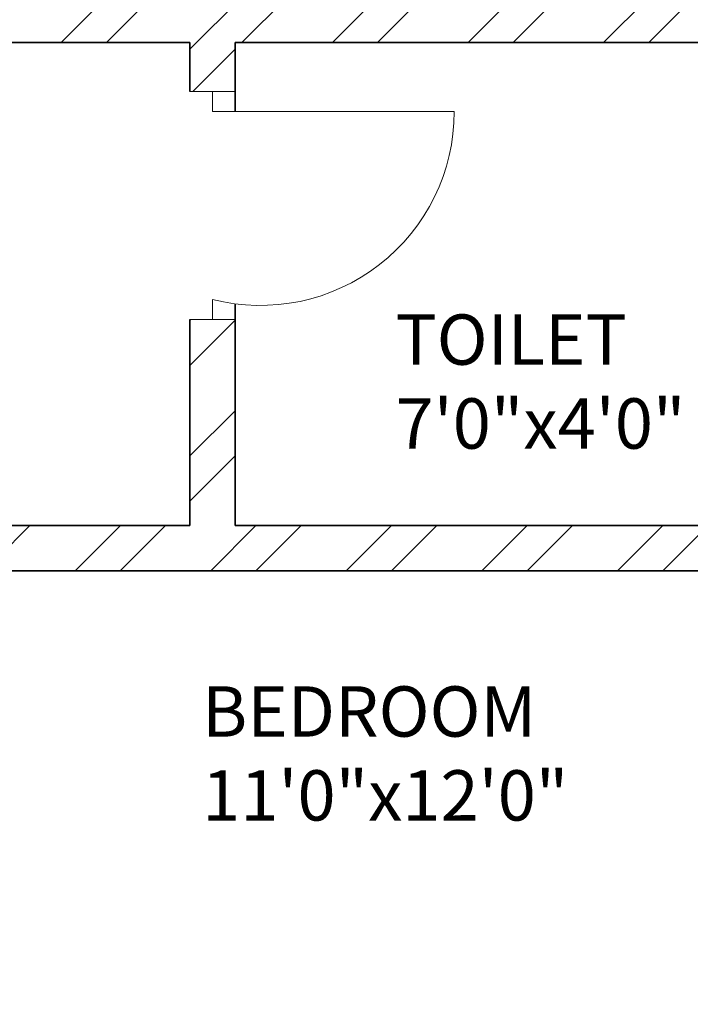
# Model space of a CAD drawing. Units: inches. Extents: x 1962 to 2771, y 1245 to 2660.
# Tile 78 of 114: x 2551 to 2618, y 2082 to 2180. Entities that reach past the tile are written whole.
import ezdxf

# ---------------------------------------------------------------- set-up
doc = ezdxf.new("R2010")
doc.units = ezdxf.units.IN
for name, color, linetype, lineweight in [('A-ANNO-DIMS', 2, 'Continuous', 18), ('A-AREA-IDEN', 7, 'Continuous', 18), ('A-DOOR', 3, 'Continuous', 18), ('A-WALL', 7, 'Continuous', 35), ('A-WALL-PATT', 252, 'Continuous', 13)]:
    doc.layers.add(name, color=color, linetype=linetype, lineweight=lineweight)
doc.styles.get("Standard").update_dxf_attribs({"font": 'arial.ttf'})
doc.dimstyles.get("Standard").update_dxf_attribs({"dimtxt": 0.18, "dimasz": 0.18, "dimexe": 0.18, "dimexo": 0.0625, "dimgap": 0.09, "dimtad": 0, "dimtih": 1, "dimtoh": 1, "dimdec": 4, "dimzin": 0, "dimdsep": 46, "dimtxsty": 'Standard', "dimcen": 0.09, "dimadec": 0, "dimazin": 0, "dimtfac": 1, "dimtdec": 4, "dimtofl": 0, "dimtmove": 0, "dimatfit": 3, "dimfxl": 1, "dimtolj": 1, "dimtzin": 0, "dimarcsym": 0})

# ---------------------------------------------------------------- blocks, each defined once
blk = doc.blocks.new('*D40')
at = {"layer": 'A-ANNO-DIMS', "color": 0, "lineweight": -2, "transparency": 16777216}
for p, q in [((2072.02, 2033.906), (2072.02, 2583.474)), ((2072.2, 2583.294), (2366.02, 2583.294)), ((2660.627, 2583.294), (2366.808, 2583.294)), ((2660.807, 2524.406), (2660.807, 2583.474))]:
    blk.add_line(p, q, dxfattribs=at)
at = {"layer": 'A-ANNO-DIMS', "color": 0, "transparency": 16777216}
for points in [[(2072.2, 2583.324), (2072.2, 2583.264), (2072.02, 2583.294)], [(2660.627, 2583.324), (2660.627, 2583.264), (2660.807, 2583.294)]]:
    blk.add_solid(points, dxfattribs=at)
at = {"layer": 'Defpoints', "color": 0, "transparency": 16777216}
for p in [(2660.807, 2583.294), (2660.807, 2524.344), (2072.02, 2033.844)]:
    blk.add_point(p, dxfattribs=at)
at = {"layer": 'A-ANNO-DIMS', "color": 0, "transparency": 16777216, "insert": (2366.414, 2583.294), "char_height": 0.18, "attachment_point": 5}
blk.add_mtext('\\A1;588.8', dxfattribs=at)

msp = doc.modelspace()

# ---------------------------------------------------------------- hatches: boundary and pattern name
at = {"layer": 'A-WALL-PATT'}
h = msp.add_hatch(dxfattribs=at)
h.set_pattern_fill('ANSI32', color=256)
h.paths.add_polyline_path([(2090.8074, 2467.3437), (2141.6481, 2467.3437), (2141.6481, 2469.5937), (2141.6481, 2471.8437), (2086.3074, 2471.8437), (2086.3074, 2422.5333), (2090.8074, 2422.5333)])
h.paths.add_polyline_path([(2282.7664, 2471.8437), (2204.8982, 2471.8437), (2204.8982, 2467.3437), (2234.8074, 2467.3437), (2234.8074, 2311.3437), (2228.7492, 2311.3437), (2228.7492, 2306.8437), (2234.8074, 2306.8437), (2331.9227, 2306.8437), (2331.9227, 2309.0937), (2331.9227, 2311.3437), (2239.3074, 2311.3437), (2239.3074, 2467.3437), (2282.7664, 2467.3437), (2282.7664, 2469.5937)])
h.paths.add_polyline_path([(2471.4531, 2519.8437), (2552.011, 2519.8437), (2564.3996, 2519.8437), (2564.3996, 2511.1389), (2568.8996, 2511.1389), (2568.8996, 2524.3437), (2466.9531, 2524.3437), (2466.9531, 2471.8437), (2450.0749, 2471.8437), (2446.4672, 2471.8437), (2446.4672, 2467.3437), (2450.0749, 2467.3437), (2475.9988, 2467.3437), (2475.9988, 2469.5937), (2475.9988, 2471.8437), (2471.4531, 2471.8437)])
h.paths.add_polyline_path([(2575.2231, 2469.5937), (2575.2231, 2471.8437), (2568.8996, 2471.8437), (2568.8996, 2487.1389), (2564.3996, 2487.1389), (2564.3996, 2471.8437), (2556.511, 2471.8437), (2499.2904, 2471.8437), (2499.2904, 2467.3437), (2507.8074, 2467.3437), (2507.8074, 2311.3437), (2414.863, 2311.3437), (2414.863, 2306.8437), (2512.3074, 2306.8437), (2517.0114, 2306.8437), (2517.0114, 2309.0937), (2517.0114, 2311.3437), (2512.3074, 2311.3437), (2512.3074, 2467.3437), (2575.2231, 2467.3437)])
h.paths.add_polyline_path([(2660.8074, 2471.8437), (2600.9602, 2471.8437), (2600.9602, 2467.3437), (2656.3074, 2467.3437), (2656.3074, 2432.5704), (2660.8074, 2432.5704)])
h.paths.add_polyline_path([(2660.8074, 2372.5704), (2656.3074, 2372.5704), (2656.3074, 2311.3437), (2600.276, 2311.3437), (2600.276, 2309.0937), (2600.276, 2306.8437), (2656.3074, 2306.8437), (2656.3074, 2296.2593), (2660.8074, 2296.2593)])
h.paths.add_polyline_path([(2572.3074, 2306.8437), (2577.1385, 2306.8437), (2577.1385, 2311.3437), (2551.082, 2311.3437), (2551.082, 2306.8437), (2567.8074, 2306.8437), (2567.8074, 2258.8437), (2540.0574, 2258.8437), (2540.0574, 2256.5937), (2540.0574, 2254.3437), (2567.8074, 2254.3437), (2656.3074, 2254.3437), (2656.3074, 2236.9085), (2660.8074, 2236.9085), (2660.8074, 2272.2593), (2656.3074, 2272.2593), (2656.3074, 2258.8437), (2572.3074, 2258.8437)])
h.paths.add_polyline_path([(2512.3074, 2254.3437), (2518.8716, 2254.3437), (2518.8716, 2256.5937), (2518.8716, 2258.8437), (2507.8074, 2258.8437), (2507.8074, 2177.8437), (2567.8074, 2177.8437), (2567.8074, 2172.9628), (2572.3074, 2172.9628), (2572.3074, 2177.8437), (2656.3074, 2177.8437), (2656.3074, 2166.4846), (2660.8074, 2166.4846), (2660.8074, 2200.9085), (2656.3074, 2200.9085), (2656.3074, 2182.3437), (2512.3074, 2182.3437)])
h.paths.add_polyline_path([(2656.3074, 2129.8437), (2572.3074, 2129.8437), (2572.3074, 2150.3044), (2570.0574, 2150.3044), (2567.8074, 2150.3044), (2567.8074, 2129.8437), (2507.8074, 2129.8437), (2507.8074, 2116.3027), (2510.0574, 2116.3027), (2512.3074, 2116.3027), (2512.3074, 2125.3437), (2567.8074, 2125.3437), (2572.3074, 2125.3437), (2656.3074, 2125.3437)])
h.paths.add_polyline_path([(2090.8074, 2362.5333), (2086.3074, 2362.5333), (2086.3074, 2298.6242), (2090.8074, 2298.6242), (2090.8074, 2306.8437), (2174.8074, 2306.8437), (2174.8074, 2286.4178), (2179.3074, 2286.4178), (2179.3074, 2306.8437), (2192.8641, 2306.8437), (2192.8641, 2309.0937), (2192.8641, 2311.3437), (2090.8074, 2311.3437)])
h.paths.add_polyline_path([(2209.156, 2258.8437), (2179.3074, 2258.8437), (2179.3074, 2263.2236), (2177.0574, 2263.2236), (2174.8074, 2263.2236), (2174.8074, 2258.8437), (2090.8074, 2258.8437), (2090.8074, 2274.6242), (2086.3074, 2274.6242), (2086.3074, 2238.2967), (2088.5574, 2238.2967), (2090.8074, 2238.2967), (2090.8074, 2254.3437), (2209.156, 2254.3437)])
h.paths.add_polyline_path([(2090.8074, 2177.8437), (2234.8074, 2177.8437), (2234.8074, 2173.1428), (2239.3074, 2173.1428), (2239.3074, 2258.8437), (2230.8442, 2258.8437), (2230.8442, 2256.5937), (2230.8442, 2254.3437), (2234.8074, 2254.3437), (2234.8074, 2182.3437), (2090.8074, 2182.3437), (2090.8074, 2202.2967), (2086.3074, 2202.2967), (2086.3074, 2140.0389), (2090.8074, 2140.0389)])
h.paths.add_polyline_path([(2090.8074, 2080.0389), (2086.3074, 2080.0389), (2086.3074, 2033.8437), (2090.8074, 2033.8437)], flags=17)
h.paths.add_polyline_path([(2244.9405, 2033.8437), (2239.3074, 2033.8437), (2239.3074, 2142.0665), (2237.2592, 2142.0665), (2234.8074, 2142.0665), (2234.8074, 2033.8437), (2090.8074, 2033.8437), (2076.5204, 2033.8437), (2072.0204, 2033.8437), (2072.0204, 2000.4493), (2076.5204, 2000.4493), (2076.5204, 2029.3437), (2090.8074, 2029.3437), (2244.9405, 2029.3437), (2244.9405, 2031.5937)])
h.paths.add_polyline_path([(2234.8074, 1933.3437), (2076.5204, 1933.3437), (2076.5204, 1952.4493), (2074.2704, 1952.4493), (2072.0204, 1952.4493), (2072.0204, 1933.3437), (2072.0204, 1928.8437), (2234.8074, 1928.8437)])
h.paths.add_polyline_path([(2090.8074, 1928.8437), (2086.3074, 1928.8437), (2086.3074, 1906.5013), (2090.8074, 1906.5013)])
h.paths.add_polyline_path([(2090.8074, 1846.5013), (2086.3074, 1846.5013), (2086.3074, 1769.9917), (2088.5574, 1769.9917), (2090.8074, 1769.9917), (2090.8074, 1780.3437), (2234.8074, 1780.3437), (2234.8074, 1708.3437), (2230.3764, 1708.3437), (2230.3764, 1703.8437), (2239.3074, 1703.8437), (2239.3074, 1792.6669), (2237.0574, 1792.6669), (2234.8074, 1792.6669), (2234.8074, 1784.8437), (2090.8074, 1784.8437)])
h.paths.add_polyline_path([(2239.3074, 1928.8437), (2244.9405, 1928.8437), (2244.9405, 1931.0937), (2244.9405, 1933.3437), (2234.8074, 1933.3437), (2234.8074, 1928.8437), (2234.8074, 1825.5949), (2239.3074, 1825.5949)])
h.paths.add_polyline_path([(2148.0425, 1649.0937), (2148.0425, 1651.3437), (2090.8074, 1651.3437), (2090.8074, 1646.8437), (2148.0425, 1646.8437)], flags=0)
h.paths.add_polyline_path([(2207.5601, 1708.3437), (2090.8074, 1708.3437), (2090.8074, 1703.8437), (2174.8074, 1703.8437), (2174.8074, 1651.3437), (2170.4457, 1651.3437), (2170.4457, 1646.8437), (2195.9924, 1646.8437), (2195.9924, 1649.0937), (2195.9924, 1651.3437), (2179.3074, 1651.3437), (2179.3074, 1703.8437), (2207.5601, 1703.8437), (2207.5601, 1706.0937)])
h.paths.add_polyline_path([(2090.8074, 1733.9917), (2086.3074, 1733.9917), (2086.3074, 1696.1032), (2088.5574, 1696.1032), (2090.8074, 1696.1032)])
h.paths.add_polyline_path([(2090.8074, 1672.1032), (2086.3074, 1672.1032), (2086.3074, 1600.3335), (2090.8074, 1600.3335)])
h.paths.add_polyline_path([(2090.8074, 1540.3335), (2086.3074, 1540.3335), (2086.3074, 1486.3437), (2139.6766, 1486.3437), (2139.6766, 1490.8437), (2090.8074, 1490.8437)])
h.paths.add_polyline_path([(2302.3876, 1490.8437), (2239.3074, 1490.8437), (2239.3074, 1646.8437), (2335.9994, 1646.8437), (2335.9994, 1651.3437), (2229.884, 1651.3437), (2229.884, 1646.8437), (2234.8074, 1646.8437), (2234.8074, 1490.8437), (2202.7103, 1490.8437), (2202.7103, 1488.5937), (2202.7103, 1486.3437), (2275.0699, 1486.3437), (2275.0699, 1475.772), (2279.5699, 1475.772), (2279.5699, 1486.3437), (2302.3876, 1486.3437)])
h.paths.add_polyline_path([(2279.5699, 1451.772), (2275.0699, 1451.772), (2275.0699, 1438.3437), (2174.8074, 1438.3437), (2174.8074, 1486.3437), (2179.7922, 1486.3437), (2179.7922, 1490.8437), (2163.3585, 1490.8437), (2163.3585, 1488.5937), (2163.3585, 1486.3437), (2170.3074, 1486.3437), (2170.3074, 1433.8437), (2279.5699, 1433.8437)])
h.paths.add_polyline_path([(2427.2363, 1490.8437), (2375.8074, 1490.8437), (2375.8074, 1646.8437), (2381.6401, 1646.8437), (2381.6401, 1651.3437), (2365.887, 1651.3437), (2365.887, 1649.0937), (2365.887, 1646.8437), (2371.3074, 1646.8437), (2371.3074, 1490.8437), (2327.5627, 1490.8437), (2327.5627, 1488.5937), (2327.5627, 1486.3437), (2371.3074, 1486.3437), (2371.3074, 1433.8437), (2375.8074, 1433.8437), (2375.8074, 1486.3437), (2427.2363, 1486.3437)])
h.paths.add_polyline_path([(2512.3074, 1646.8437), (2519.4351, 1646.8437), (2519.4351, 1649.0937), (2519.4351, 1651.3437), (2507.8074, 1651.3437), (2416.0063, 1651.3437), (2416.0063, 1649.0937), (2416.0063, 1646.8437), (2507.8074, 1646.8437), (2507.8074, 1490.8437), (2497.0532, 1490.8437), (2497.0532, 1488.5937), (2497.0532, 1486.3437), (2574.9344, 1486.3437), (2574.9344, 1476.0181), (2579.4344, 1476.0181), (2579.4344, 1486.3437), (2584.4872, 1486.3437), (2584.3074, 1490.8437), (2512.3074, 1490.8437)])
h.paths.add_polyline_path([(2470.5091, 1486.3437), (2473.9767, 1486.3437), (2473.9767, 1490.8437), (2449.6605, 1490.8437), (2449.6605, 1488.5937), (2449.6605, 1486.3437), (2466.0091, 1486.3437), (2466.0091, 1433.8437), (2470.5091, 1433.8437), (2579.4344, 1433.8437), (2579.4344, 1452.0181), (2574.9344, 1452.0181), (2574.9344, 1438.3437), (2554.5091, 1438.3437), (2470.5091, 1438.3437)])
h.paths.add_polyline_path([(2656.3074, 1490.8437), (2611.86, 1490.8437), (2611.86, 1486.3437), (2656.3074, 1486.3437)])
h.paths.add_polyline_path([(2660.8074, 1532.7007), (2658.5574, 1532.7007), (2656.3074, 1532.7007), (2656.3074, 1486.3437), (2660.8074, 1486.3437)])
h.paths.add_polyline_path([(2660.8074, 1664.9663), (2656.3074, 1664.9663), (2656.3074, 1651.3437), (2602.2313, 1651.3437), (2602.2313, 1646.8437), (2656.3074, 1646.8437), (2656.3074, 1592.7007), (2660.8074, 1592.7007)])
h.paths.add_polyline_path([(2660.8074, 1724.5221), (2656.3074, 1724.5221), (2656.3074, 1703.8437), (2542.4725, 1703.8437), (2542.4725, 1699.3437), (2567.8074, 1699.3437), (2567.8074, 1651.3437), (2552.7766, 1651.3437), (2552.7766, 1649.0937), (2552.7766, 1646.8437), (2577.2878, 1646.8437), (2577.2878, 1649.0937), (2577.2878, 1651.3437), (2572.3074, 1651.3437), (2572.3074, 1699.3437), (2656.3074, 1699.3437), (2656.3074, 1688.9663), (2660.8074, 1688.9663)])
h.paths.add_polyline_path([(2660.8074, 1880.6524), (2656.3074, 1880.6524), (2656.3074, 1832.8437), (2512.3074, 1832.8437), (2512.3074, 1837.8959), (2507.8074, 1837.8959), (2507.8074, 1828.3437), (2567.8074, 1828.3437), (2567.8074, 1804.3437), (2572.3074, 1804.3437), (2572.3074, 1828.3437), (2656.3074, 1828.3437), (2656.3074, 1818.6778), (2660.8074, 1818.6778)])
h.paths.add_polyline_path([(2660.8074, 1794.6778), (2656.3074, 1794.6778), (2656.3074, 1780.3437), (2572.3074, 1780.3437), (2572.3074, 1783.0303), (2570.0574, 1783.0303), (2567.8074, 1783.0303), (2567.8074, 1780.3437), (2507.8074, 1780.3437), (2507.8074, 1699.3437), (2517.8858, 1699.3437), (2517.8858, 1701.5937), (2517.8858, 1703.8437), (2512.3074, 1703.8437), (2512.3074, 1775.8437), (2656.3074, 1775.8437), (2656.3074, 1760.5221), (2660.8074, 1760.5221)])
h.paths.add_polyline_path([(2660.8074, 1981.3437), (2660.8074, 2020.2808), (2658.5574, 2020.2808), (2656.3074, 2020.2808), (2656.3074, 1981.3437), (2512.3074, 1981.3437), (2512.3074, 2086.6996), (2507.8074, 2086.6996), (2507.8074, 1981.3437), (2375.8074, 1981.3437), (2375.8074, 1986.8505), (2373.5574, 1986.8505), (2371.3074, 1986.8505), (2371.3074, 1973.2607), (2375.8074, 1973.2607), (2375.8074, 1976.8437), (2507.8074, 1976.8437), (2507.8074, 1865.4281), (2510.0574, 1865.4281), (2512.3074, 1865.4281), (2512.3074, 1976.8437), (2660.8074, 1976.8437)])
h.paths.add_polyline_path([(2375.8074, 1940.297), (2373.5574, 1940.297), (2371.3074, 1940.297), (2371.3074, 1933.3437), (2278.4434, 1933.3437), (2278.4434, 1928.8437), (2371.3074, 1928.8437), (2371.3074, 1651.3437), (2375.8074, 1651.3437)])
h.paths.add_polyline_path([(2660.8074, 1976.8437), (2656.3074, 1976.8437), (2656.3074, 1940.6524), (2660.8074, 1940.6524)], flags=17)
h.paths.add_polyline_path([(2660.8074, 2142.4846), (2656.3074, 2142.4846), (2656.3074, 2080.2808), (2660.8074, 2080.2808)])
h.paths.add_polyline_path([(2381.4189, 2311.3437), (2375.8074, 2311.3437), (2375.8074, 2467.3437), (2424.7242, 2467.3437), (2424.7242, 2469.5937), (2424.7242, 2471.8437), (2375.8074, 2471.8437), (2375.8074, 2524.3437), (2371.3074, 2524.3437), (2371.3074, 2471.8437), (2307.2097, 2471.8437), (2307.2097, 2467.3437), (2371.3074, 2467.3437), (2371.3074, 2311.3437), (2366.8901, 2311.3437), (2366.8901, 2306.8437), (2371.3074, 2306.8437), (2371.3074, 2033.8437), (2279.6589, 2033.8437), (2279.6589, 2029.3437), (2371.3074, 2029.3437), (2371.3074, 2014.2598), (2375.8074, 2014.2598), (2375.8074, 2306.8437), (2381.4189, 2306.8437)])
h.paths.add_polyline_path([(2263.3074, 2524.3437), (2170.3074, 2524.3437), (2170.3074, 2519.8437), (2170.3074, 2471.8437), (2165.0312, 2471.8437), (2165.0312, 2467.3437), (2179.6721, 2467.3437), (2179.6721, 2469.5161), (2179.6721, 2471.8437), (2174.8074, 2471.8437), (2174.8074, 2519.8437), (2258.8074, 2519.8437), (2258.8074, 2511.6436), (2263.3074, 2511.6436)])
h.paths.add_polyline_path([(2245.0232, 1361.4123), (2492.9468, 1361.4123), (2492.9468, 1398.505), (2245.0232, 1398.505)], flags=9)
h.paths.add_polyline_path([(2388.1434, 2086.6936), (2425.0704, 2086.6936), (2425.0704, 2105.3509), (2388.1434, 2105.3509)], flags=9)
h.paths.add_polyline_path([(2404.922, 2242.6744), (2445.7337, 2242.6744), (2445.7337, 2261.3318), (2404.922, 2261.3318)], flags=9)
h.paths.add_polyline_path([(2269.4107, 2156.7935), (2306.3378, 2156.7935), (2306.3378, 2175.4508), (2269.4107, 2175.4508)], flags=9)
h.paths.add_polyline_path([(2269.3277, 2233.4343), (2306.2547, 2233.4343), (2306.2547, 2252.0917), (2269.3277, 2252.0917)], flags=9)
h.paths.add_polyline_path([(2431.6052, 2320.6922), (2470.4456, 2320.6922), (2470.4456, 2339.3495), (2431.6052, 2339.3495)], flags=25)
h.paths.add_polyline_path([(2249.6902, 2315.7608), (2288.5306, 2315.7608), (2288.5306, 2334.4182), (2249.6902, 2334.4182)], flags=25)
h.paths.add_polyline_path([(2096.9301, 2314.3181), (2135.7704, 2314.3181), (2135.7704, 2332.9755), (2096.9301, 2332.9755)], flags=25)
h.paths.add_polyline_path([(2134.3475, 2285.7089), (2161.4655, 2285.7089), (2161.4655, 2304.3662), (2134.3475, 2304.3662)], flags=9)
h.paths.add_polyline_path([(2126.5155, 2209.4076), (2159.9227, 2209.4076), (2159.9227, 2228.065), (2126.5155, 2228.065)], flags=25)
h.paths.add_polyline_path([(2110.5753, 2141.5299), (2149.4157, 2141.5299), (2149.4157, 2160.1872), (2110.5753, 2160.1872)], flags=25)
h.paths.add_polyline_path([(2249.8618, 1968.3317), (2286.3966, 1968.3317), (2286.3966, 1986.989), (2249.8618, 1986.989)], flags=9)
h.paths.add_polyline_path([(2395.9507, 1777.0051), (2436.7624, 1777.0051), (2436.7624, 1795.6625), (2395.9507, 1795.6625)], flags=9)
h.paths.add_polyline_path([(2398.5259, 1888.5651), (2435.0062, 1888.5651), (2435.0062, 1907.2224), (2398.5259, 1907.2224)], flags=25)
h.paths.add_polyline_path([(2259.3506, 1728.3559), (2296.2776, 1728.3559), (2296.2776, 1747.0132), (2259.3506, 1747.0132)], flags=9)
h.paths.add_polyline_path([(2271.3698, 1845.268), (2308.2968, 1845.268), (2308.2968, 1863.9253), (2271.3698, 1863.9253)], flags=9)
h.paths.add_polyline_path([(2120.9355, 1786.3027), (2159.7759, 1786.3027), (2159.7759, 1804.9601), (2120.9355, 1804.9601)], flags=25)
h.paths.add_polyline_path([(2121.3164, 1732.1043), (2154.7236, 1732.1043), (2154.7236, 1750.7616), (2121.3164, 1750.7616)], flags=25)
h.paths.add_polyline_path([(2118.3706, 1678.8997), (2147.5282, 1678.8997), (2147.5282, 1697.557), (2118.3706, 1697.557)], flags=25)
h.paths.add_polyline_path([(2385.9227, 1493.557), (2424.763, 1493.557), (2424.763, 1512.2143), (2385.9227, 1512.2143)], flags=25)
h.paths.add_polyline_path([(2248.7058, 1500.0256), (2287.5462, 1500.0256), (2287.5462, 1518.6829), (2248.7058, 1518.6829)], flags=25)
h.paths.add_polyline_path([(2104.1669, 1617.3771), (2143.0073, 1617.3771), (2143.0073, 1636.0344), (2104.1669, 1636.0344)], flags=9)
h.paths.add_polyline_path([(2096.0714, 1447.8824), (2137.3845, 1447.8824), (2137.3845, 1458.1859), (2096.0714, 1458.1859)], flags=9)
h.paths.add_polyline_path([(2180.6114, 1440.325), (2209.7689, 1440.325), (2209.7689, 1458.9823), (2180.6114, 1458.9823)], flags=25)
h.paths.add_polyline_path([(2316.1698, 1447.9637), (2357.4829, 1447.9637), (2357.4829, 1458.2673), (2316.1698, 1458.2673)], flags=9)
h.paths.add_polyline_path([(2397.6187, 1447.9637), (2438.9318, 1447.9637), (2438.9318, 1458.2673), (2397.6187, 1458.2673)], flags=9)
h.paths.add_polyline_path([(2473.0778, 1439.5953), (2502.2354, 1439.5953), (2502.2354, 1458.2527), (2473.0778, 1458.2527)], flags=25)
h.paths.add_polyline_path([(2589.7027, 1447.8819), (2631.0158, 1447.8819), (2631.0158, 1458.1855), (2589.7027, 1458.1855)], flags=9)
h.paths.add_polyline_path([(2522.4009, 1497.5285), (2561.2413, 1497.5285), (2561.2413, 1516.1859), (2522.4009, 1516.1859)], flags=25)
h.paths.add_polyline_path([(2579.6565, 1671.3482), (2608.8141, 1671.3482), (2608.8141, 1690.0056), (2579.6565, 1690.0056)], flags=25)
h.paths.add_polyline_path([(2544.7038, 1725.5064), (2578.1111, 1725.5064), (2578.1111, 1744.1637), (2544.7038, 1744.1637)], flags=25)
h.paths.add_polyline_path([(2578.1191, 1807.472), (2607.2766, 1807.472), (2607.2766, 1826.1293), (2578.1191, 1826.1293)], flags=25)
h.paths.add_polyline_path([(2595.0614, 1835.1839), (2633.9018, 1835.1839), (2633.9018, 1853.8413), (2595.0614, 1853.8413)], flags=25)
h.paths.add_polyline_path([(2567.0097, 2097.7035), (2605.8501, 2097.7035), (2605.8501, 2116.3609), (2567.0097, 2116.3609)], flags=9)
h.paths.add_polyline_path([(2586.644, 2134.6454), (2615.8015, 2134.6454), (2615.8015, 2153.3027), (2586.644, 2153.3027)], flags=9)
h.paths.add_polyline_path([(2544.6185, 2212.6783), (2578.0258, 2212.6783), (2578.0258, 2231.3356), (2544.6185, 2231.3356)], flags=25)
h.paths.add_polyline_path([(2577.0273, 2256.9023), (2606.1849, 2256.9023), (2606.1849, 2275.5597), (2577.0273, 2275.5597)], flags=24)
h.paths.add_polyline_path([(2605.2683, 2315.2821), (2644.1087, 2315.2821), (2644.1087, 2333.9395), (2605.2683, 2333.9395)], flags=25)
h.paths.add_polyline_path([(2583.1244, 2496.1815), (2624.4375, 2496.1815), (2624.4375, 2506.4851), (2583.1244, 2506.4851)], flags=9)
h.paths.add_polyline_path([(2474.761, 2497.0823), (2503.9185, 2497.0823), (2503.9185, 2515.7397), (2474.761, 2515.7397)], flags=25)
h.paths.add_polyline_path([(2387.5787, 2494.2563), (2428.902, 2494.2563), (2428.902, 2504.5598), (2387.5787, 2504.5598)], flags=9)
h.paths.add_polyline_path([(2300.1657, 2500.1564), (2341.4788, 2500.1564), (2341.4788, 2510.46), (2300.1657, 2510.46)], flags=25)
h.paths.add_polyline_path([(2176.8589, 2497.5843), (2206.0165, 2497.5843), (2206.0165, 2516.2416), (2176.8589, 2516.2416)], flags=25)
h.paths.add_polyline_path([(2097.4668, 2494.9762), (2138.7799, 2494.9762), (2138.7799, 2505.2798), (2097.4668, 2505.2798)], flags=9)

# ---------------------------------------------------------------- linework, layer by layer
at = {"layer": 'A-DOOR'}
for p, q in [((2567.8074, 2172.9628), (2572.3074, 2172.9628)), ((2572.3074, 2172.9628), (2570.0574, 2172.9628)), ((2570.0574, 2172.9628), (2570.0574, 2170.9628)), ((2570.0574, 2170.9628), (2594.0574, 2170.9628)), ((2570.0574, 2150.3044), (2570.0574, 2152.3044)), ((2567.8074, 2150.3044), (2572.3074, 2150.3044)), ((2572.3074, 2150.3044), (2570.0574, 2150.3044))]:
    msp.add_line(p, q, dxfattribs=at)
msp.add_arc((2574.8046, 2170.9628), 19.2528, 255.725354, 0, dxfattribs=at)
at = {"layer": 'A-WALL'}
for p, q in [((2567.8074, 2177.8437), (2507.8074, 2177.8437)), ((2567.8074, 2172.9628), (2567.8074, 2177.8437)), ((2656.3074, 2177.8437), (2572.3074, 2177.8437)), ((2656.3074, 2177.8437), (2572.3074, 2177.8437)), ((2572.3074, 2177.8437), (2572.3074, 2170.9628)), ((2572.3074, 2151.8726), (2572.3074, 2129.8437)), ((2567.8074, 2129.8437), (2567.8074, 2150.3044)), ((2567.8074, 2129.8437), (2507.8074, 2129.8437)), ((2572.3074, 2129.8437), (2656.3074, 2129.8437)), ((2567.8074, 2125.3437), (2512.3074, 2125.3437)), ((2572.3074, 2125.3437), (2567.8074, 2125.3437)), ((2656.3074, 2125.3437), (2572.3074, 2125.3437))]:
    msp.add_line(p, q, dxfattribs=at)

# ---------------------------------------------------------------- texts
at = {"layer": 'A-AREA-IDEN', "char_height": 5, "attachment_point": 1}
for s, width, insert in [('TOILET\\P7\'0"x4\'0"', 97.357493, (2588.2248, 2150.8181)), ('BEDROOM\\P11\'0"x12\'0"', 117.696406, (2569.0203, 2113.8762))]:
    msp.add_mtext_dynamic_manual_height_columns(s, width=width, gutter_width=12.5, heights=[0], dxfattribs=dict(at, insert=insert))

# ---------------------------------------------------------------- dimensions: what is measured, and where the dimension line sits
at = {"layer": 'A-ANNO-DIMS'}
dim = msp.add_linear_dim(base=(2660.8074, 2583.2937), p1=(2072.0204, 2033.8437), p2=(2660.8074, 2524.3437), dimstyle='Standard', override={"dimdec": 1, "dimlfac": 1, "dimrnd": 0, "dimzin": 0, "dimdsep": 46, "dimlunit": 2}, dxfattribs=at)
dim.commit()
dim.dimension.update_dxf_attribs({"geometry": '*D40', "text_midpoint": (2366.4139, 2583.2937)})

doc.saveas('drawing.dxf')
